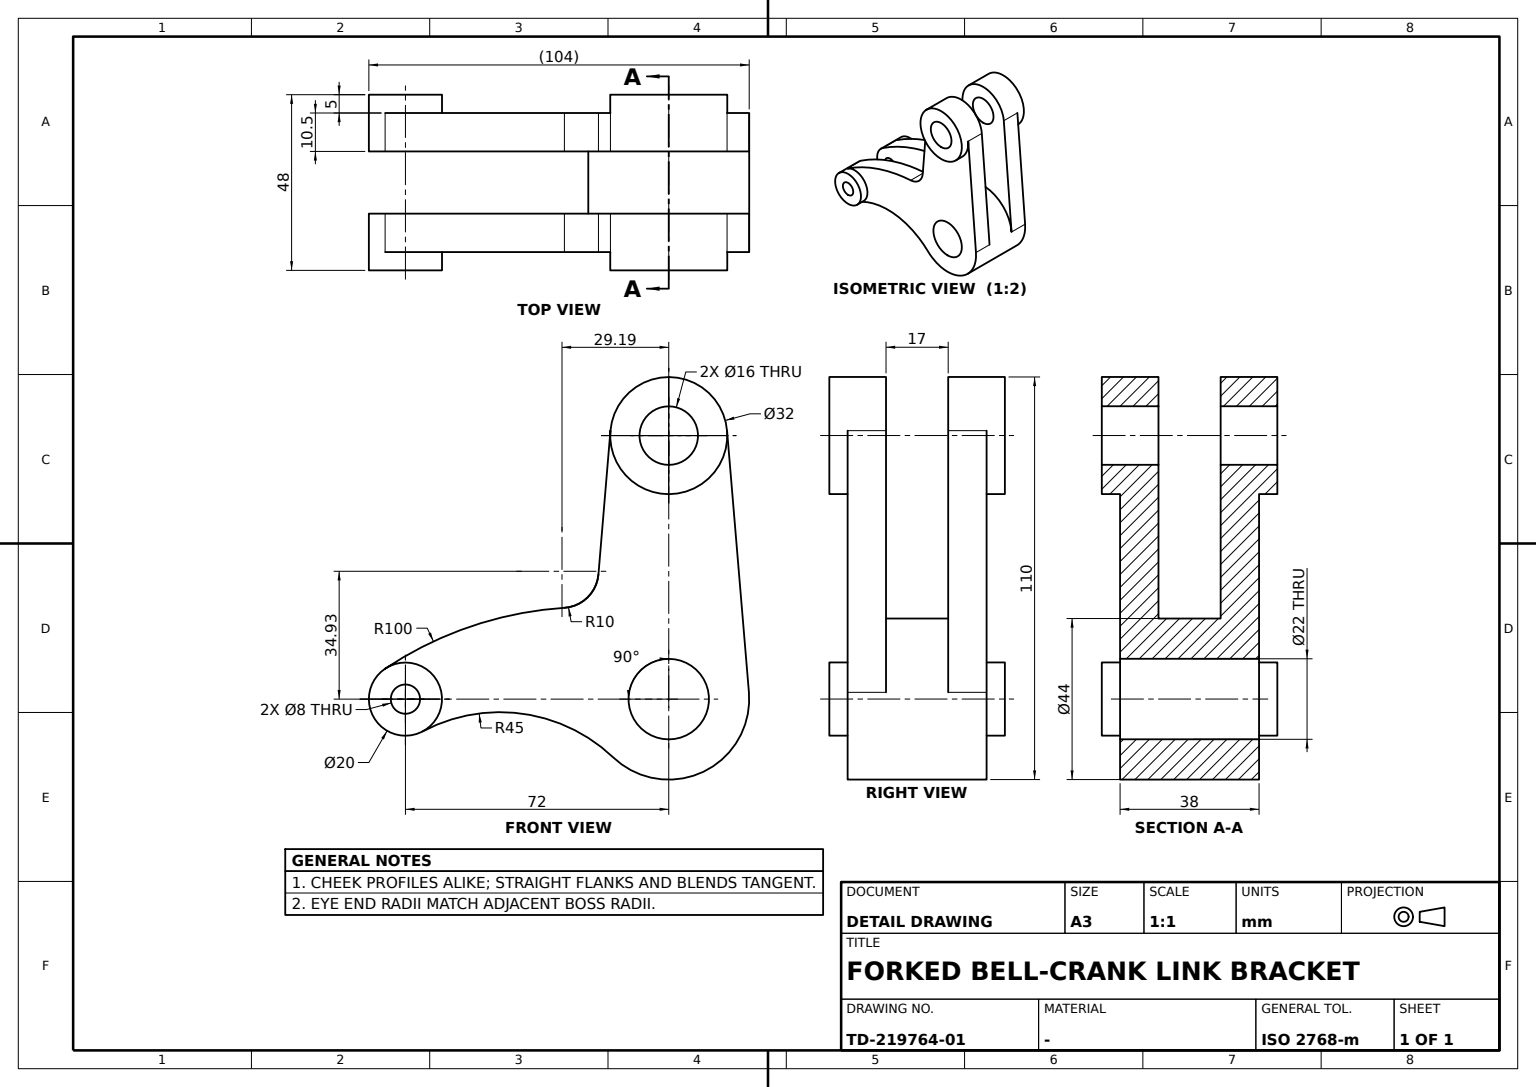
CATIA V5 part; units mm, degrees
sketch "Sketch1" plane through (0, 0, 0) normal (1, 0, 0) x (0, 1, 0)
  circle A0 centre (0, 0) radius 22
  circle A1 centre (0, 0) radius 11
  point P0 (0, -11)
  dimension "radius A0" = 22
  dimension "radius A1" = 11
  constraint coincidence A1 P0
  constraint coincidence P0 y-axis
extrude "Pad1" add sketch "Sketch1" along normal mid plane 38
sketch "Sketch2" plane through (19, 0, 0) normal (1, 0, 0) x (0, 1, 0)
  arc A0 (77.5553, 8.315) -> (67.303, -8.8283) centre (72, 0) ccw
  point P0 (72, 0)
  arc A1 (19.2248, 34.0968) -> (28.5366, 24.9514) centre (29.19, 34.93) ccw
  point P1 (29.19, 34.93)
  arc A2 (-15.9443, 73.3333) -> (15.9444, 73.3331) centre (0, 72) ccw
  point P2 (0, 72)
  circle A3 centre (0, 0) radius 22 construction
  arc A4 (15.1592, -15.9436) -> (-21.9235, 1.8333) centre (0, 0) ccw
  line L0 (-21.9235, 1.8333) -> (-15.9443, 73.3333)
  point P3 (-21.9235, 1.8333)
  line L1 (15.9444, 73.3331) -> (19.2248, 34.0968)
  arc A5 (15.1592, -15.9436) -> (67.303, -8.8283) centre (46.1667, -48.5555) cw
  point P4 (15.1592, -15.9436)
  arc A6 (28.5366, 24.9514) -> (77.5553, 8.315) centre (22.0027, -74.8349) cw
  dimension "radius A0" = 10
  dimension "distance P0 y axis" = 72
  dimension "radius A2" = 16
  dimension "radius A1" = 10
  dimension "distance x axis P1" = 34.93
  dimension "distance P1 y axis" = 29.19
  dimension "distance x axis P2" = 72
  dimension "radius A5" = 45
  dimension "radius A6" = 100
  constraint coincidence P0 x-axis
  constraint coincidence P2 y-axis
  constraint coincidence A3 P3
  constraint coincidence P4 A3
  constraint tangency L0 A3
  constraint tangency L0 A2
  constraint tangency L1 A2
  constraint tangency L1 A1
  constraint tangency A5 A3
  constraint tangency A5 A0
  constraint tangency A1 A6
  constraint tangency A6 A0
extrude "Pad2" add sketch "Sketch2" against normal blind 10.5
mirror "Mirror1" about plane through (0, 0, 0) normal (1, 0, 0) of "Pad2"
sketch "Sketch3" plane through (19, 0, 0) normal (1, 0, 0) x (0, 1, 0)
  circle A0 centre (0, 72) radius 16
  point P0 (0, 72)
  point P1 (0, 56)
  arc A1 (-15.9443, 73.3333) -> (15.9444, 73.3331) centre (0, 72) ccw construction
  arc A2 (-15.9443, 73.3333) -> (15.9444, 73.3331) centre (0, 72) ccw construction
  circle A3 centre (0, 72) radius 8
  circle A4 centre (72, 0) radius 10
  arc A5 (77.5553, 8.315) -> (67.303, -8.8283) centre (72, 0) ccw construction
  circle A6 centre (72, 0) radius 4
  dimension "radius A3" = 8
  dimension "radius A6" = 4
  constraint coincidence P0 y-axis
  constraint coincidence A0 P1
  constraint coincidence P1 y-axis
  constraint coincidence A0 A2
  constraint coincidence A4 A5
  constraint concentricity A0 A1
extrude "Pad3" add sketch "Sketch3" along normal blind 5 and the other way blind 10.5
mirror "Mirror2" about plane through (0, 0, 0) normal (1, 0, 0) of "Pad3"
